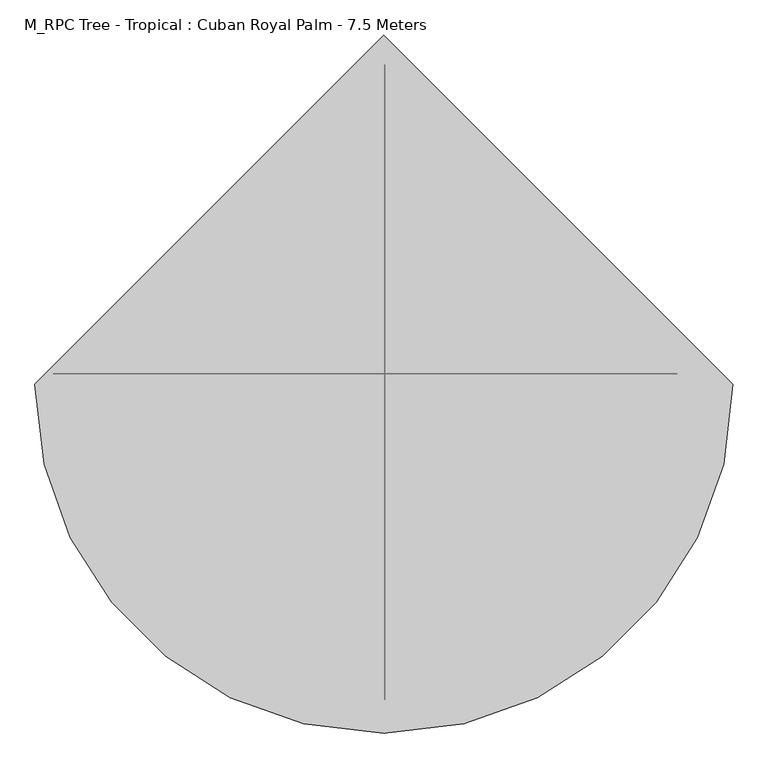
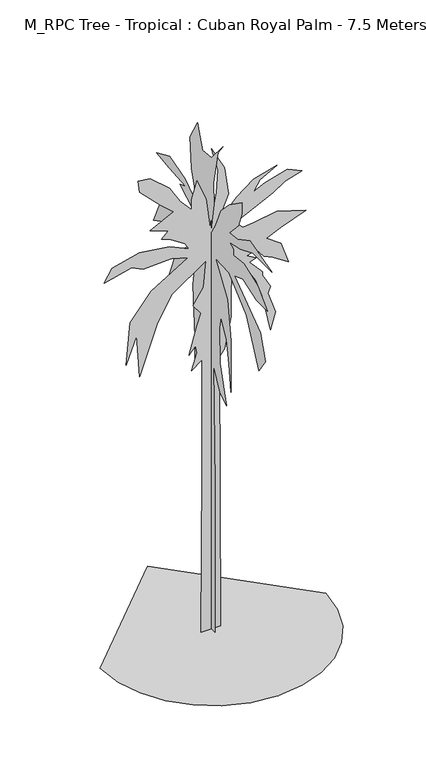
"""IFC4 building model written with IfcOpenShell, lengths in millimetres: geographic element geometry, M_RPC Tree - Tropical : Cuban Royal Palm - 7.5 Meters."""

from ifc_helpers import new_model, si_unit, origin, place, context, project, spatial, triangles, source, transform, mapped, element, save


def m_rpc_tree_tropical_cuban_royal_palm_7_5_meters_87faf919(model_context):
    return source(origin(), model_context, "Body", "Tessellation", [
        triangles([(-53.3295255, -0.0172155, 0.0009289), (-147.4824313, -0.0172239, 0.000933), (-128.6516948, -0.0176557, 2455.3626274), (-128.6514496, -0.0179554, 4131.270797), (-279.2955611, -0.0179286, 4018.2960068), (-203.9743774, -0.0179756, 4263.0955994), (-222.804369, -0.017995, 4376.0706802), (-316.9580152, -0.0179707, 4263.0955994), (-203.9741412, -0.0180497, 4677.3703125), (-147.482177, -0.0180825, 4846.8451424), (-260.4655695, -0.0181045, 4997.4949585), (-109.8212218, -0.0181515, 5223.4445389), (-72.1600077, -0.0182238, 5618.8942383), (-561.755246, -0.0181418, 5279.9445786), (-768.8900591, -0.0180688, 4922.1699051), (-1032.519825, -0.017926, 4187.7708366), (-1070.1798082, -0.0180388, 4828.0201286), (-1220.8246101, -0.0179615, 4432.5704292), (-1164.3346716, -0.0180751, 5053.9699997), (-863.0449951, -0.0181556, 5430.5946854), (-335.7879704, -0.0182359, 5750.7193314), (-580.5852376, -0.0182387, 5826.0443848), (-976.027343, -0.018218, 5807.1943726), (-1145.5022455, -0.0182241, 5882.5188446), (-1540.9443146, -0.0181899, 5788.3693588), (-1427.9619667, -0.0182286, 5976.6689117), (-1032.519825, -0.0182627, 6070.8439774), (-599.4152292, -0.0182715, 6014.3439377), (-316.9580152, -0.0182603, 5882.5188446), (-373.4504608, -0.0182746, 5976.6689117), (-599.4152292, -0.0182917, 6127.3190186), (-712.4001205, -0.0182935, 6164.9940445), (-618.247728, -0.0183145, 6259.1435303), (-881.8749504, -0.0183198, 6353.2935974), (-542.9252907, -0.0183649, 6522.768718), (-731.2301485, -0.018387, 6692.2432571), (-1032.519825, -0.0184277, 6993.5428894), (-1051.3497803, -0.0184571, 7163.0180099), (-881.8749504, -0.0184612, 7144.1679977), (-599.4152292, -0.0184298, 6899.3678238), (-448.7703547, -0.0183926, 6654.5682312), (-279.2955611, -0.0183663, 6466.2686783), (-279.2955611, -0.0183932, 6616.9182037), (-203.9741412, -0.0184437, 6880.5433914), (-72.1600077, -0.0183922, 6560.4181641), (-15.6683375, -0.0183139, 6108.4940048), (78.4845898, -0.0184055, 6598.09319), (97.3153263, -0.018467, 6937.0428497), (3.162393, -0.0185268, 7294.8175232), (191.4682185, -0.0184711, 6937.0428497), (247.9601737, -0.0183995, 6522.768718), (78.4845898, -0.018318, 6108.4940048), (360.9438114, -0.0183876, 6428.6186508), (605.7410786, -0.0184319, 6616.9182037), (944.6906656, -0.0184636, 6711.0682709), (699.8934711, -0.0184293, 6579.2681763), (605.7410786, -0.0183983, 6428.6186508), (775.2158358, -0.0184191, 6503.9437042), (1095.3355402, -0.01845, 6598.09319), (1302.4728241, -0.0184422, 6503.9437042), (1057.6755569, -0.018418, 6428.6186508), (888.2007271, -0.0183904, 6315.6185715), (342.1138561, -0.0183194, 6051.9939651), (455.0962403, -0.0183041, 5939.0188843), (605.7410786, -0.0183141, 5957.843898), (944.6906656, -0.018339, 6014.3439377), (1358.9653061, -0.0183335, 5882.5188446), (1001.1831476, -0.0182943, 5750.7193314), (794.0458637, -0.0182684, 5656.5692642), (1001.1831476, -0.0182506, 5505.9197388), (1114.1654955, -0.0181983, 5185.7950928), (888.2007271, -0.0182153, 5336.4446182), (756.3858805, -0.0182197, 5392.9196594), (605.7410786, -0.0182467, 5581.2442108), (605.7410786, -0.0182366, 5524.7447525), (511.588686, -0.0182258, 5487.094725), (643.4009892, -0.0182181, 5411.7696716), (549.2486329, -0.0182072, 5374.0946457), (737.5559252, -0.0181784, 5166.970079), (737.5559252, -0.0181683, 5110.4700394), (850.538273, -0.0181362, 4903.3448914), (812.8783625, -0.0181177, 4809.1951149), (925.8607103, -0.0180654, 4489.0704689), (850.538273, -0.0180184, 4244.2708763), (737.5559252, -0.0181111, 4790.3451027), (643.4009892, -0.0181575, 5072.8200119), (473.9261956, -0.0182006, 5355.269632), (304.4513658, -0.0182066, 5430.5946854), (285.6213741, -0.0181385, 5053.9699997), (285.6213741, -0.0180644, 4639.720285), (191.4682185, -0.0179795, 4187.7708366), (116.1458085, -0.0179593, 4093.6207695), (134.9762906, -0.0172295, 0.0009206), (0.1930215, 88.1876585, 0.0004872), (0.1930211, 161.0565937, 0.0005002), (0.1930215, 161.0565937, 1798.0107456), (0.1930235, 142.8396097, 4220.8958496), (0.1930219, 215.7080362, 4111.5958351), (0.1930238, 397.879602, 3729.0212219), (0.1930224, 397.879602, 4184.4707474), (0.1930226, 452.5320436, 4949.5949753), (0.1930212, 379.6621093, 5477.8947052), (0.1930204, 525.3994709, 5313.9198303), (0.1930227, 780.4417522, 4785.6201004), (0.1930231, 1071.9164028, 4421.295536), (0.193021, 1290.521228, 4075.1710236), (0.1930224, 1035.4814901, 4767.4203392), (0.193022, 871.5265995, 5168.1950043), (0.193022, 507.1819782, 5532.5442764), (0.1930205, 671.1367962, 5496.0947571), (0.1930222, 889.7440922, 5477.8947052), (0.1930219, 1090.1338955, 5514.3192261), (0.1930219, 1436.2610241, 5332.1448807), (0.1930208, 1254.0887135, 5732.9192551), (0.1930227, 1053.6989101, 5732.9192551), (0.1930224, 980.8290121, 6042.618956), (0.1930219, 634.7043543, 5969.7437531), (0.1930206, 416.0970946, 6079.0440582), (0.1930204, 780.4417522, 6279.443454), (0.1930236, 634.7043543, 6334.0936066), (0.1930213, 1035.4814901, 6370.5187088), (0.193023, 1363.3911987, 6406.9688095), (0.1930222, 1035.4814901, 6552.6936356), (0.193022, 652.921847, 6443.3933304), (0.1930203, 343.2271603, 6224.7938828), (0.1930224, 488.967029, 6698.4434601), (0.1930226, 525.3994709, 7153.8679871), (0.1930219, 343.2271603, 7481.7677399), (0.1930226, 306.794682, 7372.4674347), (0.1930225, 215.7080362, 7135.6429367), (0.1930209, -2.898197, 7153.8679871), (0.1930232, -294.3722026, 7499.9927902), (0.1930217, -166.8530786, 7336.0429138), (0.1930211, -57.549694, 6807.7431839), (0.193021, -75.7669232, 6498.043483), (0.1930205, 15.3189596, 5987.9688034), (0.1930237, -112.2016361, 6188.343782), (0.1930209, -239.7217594, 6498.043483), (0.1930209, -458.3270388, 6716.643512), (0.1930205, -768.0192547, 6935.2679581), (0.1930205, -768.0192547, 6771.2930832), (0.1930212, -676.9343348, 6534.4935837), (0.1930204, -458.3270388, 6297.6685043), (0.1930231, -658.7168421, 6315.8685562), (0.1930203, -968.409058, 6479.8184326), (0.193022, -1514.9259899, 6334.0936066), (0.1930214, -1041.278956, 6334.0936066), (0.1930223, -731.5867401, 6206.5688324), (0.1930212, -458.3270388, 6151.9186798), (0.1930219, -549.4144658, 6097.2691086), (0.1930215, -549.4144658, 6006.1938538), (0.1930218, -822.67166, 6042.618956), (0.1930224, -1168.7988613, 5915.0941818), (0.193023, -1405.6210339, 5678.2691025), (0.1930208, -1132.363876, 5678.2691025), (0.1930229, -786.2367474, 5787.5694077), (0.1930214, -585.8494148, 5714.7192032), (0.1930226, -1223.4513393, 5241.0696259), (0.1930224, -1350.971172, 4876.720063), (0.1930228, -1187.0162813, 4639.8952744), (0.1930223, -877.3241381, 5295.7197784), (0.1930226, -440.1120532, 5678.2691025), (0.1930235, -112.2016361, 5696.4941528), (0.1930228, -403.6771042, 5241.0696259), (0.1930226, -494.7619878, 4676.3203766), (0.1930204, -494.7619878, 3892.9960968), (0.1930225, -440.1120532, 4293.7707619), (0.1930215, -385.4596115, 4621.6705147), (0.1930212, -239.7217594, 4876.720063), (0.1930219, -203.2873009, 4694.5454269), (0.1930229, -221.504521, 4166.245697), (0.1930203, -385.4596115, 3619.7214981), (0.1930216, -221.504521, 3729.0212219), (0.1930209, -57.549694, 4038.7209229), (0.1930231, -93.9844068, 2253.4402142), (0.1930206, -93.9844068, 0.0004546), (-1626.8666862, -48.3554514, 0.0005339), (-1583.9693047, -420.1520797, 0.0004655), (-1461.7994362, -761.5892693, 0.0003991), (-1270.1396233, -1062.88396, 0.0003369), (-1018.7723356, -1314.2511749, 0.0002809), (-717.4776449, -1505.9109879, 0.0002335), (-376.0429261, -1628.0808563, 0.0001967), (-4.2444496, -1670.9783833, 0.0001728), (367.5538004, -1628.0808563, 0.0001642), (708.9884102, -1505.9109879, 0.0001711), (1010.2831009, -1314.2511749, 0.0001922), (1261.6503159, -1062.88396, 0.0002262), (1453.3101288, -761.5892693, 0.0002717), (1575.4799973, -420.1520797, 0.0003274), (1618.3775242, -48.3554514, 0.000392), (-4.2447494, 1574.2659725, 0.000298)], [[54, 55, 56], [48, 49, 50], [17, 18, 19], [15, 16, 17], [7, 8, 9], [83, 84, 85], [82, 83, 85], [4, 5, 6], [70, 71, 72], [66, 67, 68], [43, 44, 45], [59, 60, 61], [24, 25, 26], [24, 26, 27], [33, 34, 35], [76, 77, 78], [58, 59, 61], [58, 61, 62], [31, 32, 33], [42, 43, 45], [42, 45, 46], [37, 38, 39], [54, 56, 57], [53, 54, 57], [23, 24, 27], [23, 27, 28], [22, 23, 28], [22, 28, 29], [21, 22, 29], [58, 62, 63], [57, 58, 63], [53, 57, 63], [52, 53, 63], [36, 37, 39], [36, 39, 40], [36, 40, 41], [35, 36, 41], [35, 41, 42], [69, 70, 72], [69, 72, 73], [69, 73, 74], [65, 66, 68], [65, 68, 69], [65, 69, 74], [64, 65, 74], [47, 48, 50], [47, 50, 51], [46, 47, 51], [46, 51, 52], [33, 35, 42], [82, 85, 86], [81, 82, 86], [80, 81, 86], [33, 42, 46], [31, 33, 46], [30, 31, 46], [29, 30, 46], [15, 17, 19], [15, 19, 20], [14, 15, 20], [14, 20, 21], [13, 14, 21], [92, 93, 1], [92, 1, 2], [92, 2, 3], [92, 3, 4], [80, 86, 87], [79, 80, 87], [78, 79, 87], [76, 78, 87], [76, 87, 88], [13, 21, 29], [13, 29, 46], [13, 46, 52], [13, 52, 63], [13, 63, 64], [13, 64, 74], [13, 74, 75], [13, 75, 76], [13, 76, 88], [12, 13, 88], [12, 88, 89], [11, 12, 89], [10, 11, 89], [10, 89, 90], [9, 10, 90], [9, 90, 91], [7, 9, 91], [6, 7, 91], [4, 6, 91], [92, 4, 91], [131, 132, 133], [165, 166, 167], [105, 106, 107], [145, 146, 147], [165, 167, 168], [98, 99, 100], [131, 133, 134], [121, 122, 123], [104, 105, 107], [112, 113, 114], [171, 172, 173], [171, 173, 174], [153, 154, 155], [127, 128, 129], [118, 119, 120], [112, 114, 115], [139, 140, 141], [139, 141, 142], [159, 160, 161], [158, 159, 161], [157, 158, 161], [157, 161, 162], [104, 107, 108], [103, 104, 108], [103, 108, 109], [102, 103, 109], [127, 129, 130], [121, 123, 124], [120, 121, 124], [120, 124, 125], [118, 120, 125], [153, 155, 156], [152, 153, 156], [151, 152, 156], [151, 156, 157], [126, 127, 130], [145, 147, 148], [144, 145, 148], [144, 148, 149], [143, 144, 149], [139, 142, 143], [138, 139, 143], [137, 138, 143], [137, 143, 149], [175, 176, 94], [175, 94, 95], [175, 95, 96], [175, 96, 97], [174, 175, 97], [111, 112, 115], [115, 116, 117], [111, 115, 117], [110, 111, 117], [109, 110, 117], [165, 168, 169], [164, 165, 169], [130, 131, 134], [126, 130, 134], [126, 134, 135], [125, 126, 135], [125, 135, 136], [118, 125, 136], [151, 157, 162], [171, 174, 97], [170, 171, 97], [109, 117, 118], [109, 118, 136], [102, 109, 136], [97, 98, 100], [97, 100, 101], [170, 97, 101], [169, 170, 101], [169, 101, 102], [164, 169, 102], [163, 164, 102], [163, 102, 136], [151, 162, 163], [151, 163, 136], [151, 136, 137], [151, 137, 149], [151, 149, 150], [191, 192, 177], [190, 191, 177], [190, 177, 178], [189, 190, 178], [189, 178, 179], [189, 179, 180], [188, 189, 180], [187, 188, 180], [187, 180, 181], [187, 181, 182], [187, 182, 183], [187, 183, 184], [187, 184, 185], [187, 185, 186]], closed=False),
    ])


if __name__ == "__main__":
    model = new_model("IFC4")
    model_context = context("Model", 3, world=origin())
    ifc_project = project(units=[si_unit("LENGTHUNIT", "METRE", prefix="MILLI")], contexts=[model_context])
    site = spatial("IfcSite", under=ifc_project)
    building = spatial("IfcBuilding", under=site)
    placement = place(None, origin())
    m_rpc_tree_tropical_cuban_royal_palm_7_5_meters_shape = m_rpc_tree_tropical_cuban_royal_palm_7_5_meters_87faf919(model_context)
    element("IfcGeographicElement", 1, ObjectType="M_RPC Tree - Tropical : Cuban Royal Palm - 7.5 Meters", at=placement, inside=building, context=model_context, shape_type="MappedRepresentation", body=[
        mapped(m_rpc_tree_tropical_cuban_royal_palm_7_5_meters_shape, transform((0.0, 0.0, 0.0), x_axis=(1.0, 0.0, 0.0), y_axis=(0.0, 1.0, 0.0), z_axis=(0.0, 0.0, 1.0))),
    ])
    save(model, "model.ifc")

# Revit data of these elements
# Type "M_RPC Tree - Tropical : Cuban Royal Palm - 7.5 Meters"
#   built-in parameter 1005198 = "{2, 15},{39, RPC-16-FVGV-NKG0-7NHH-C000-ST1L-LVER-AU},{1, 0},{1, 0},{2, 35},{1, 8},{5, Color},{1, 0},{1, 0},{3, 0.8},{3, 0.8},{3, 0.8},{1, 8},{7, BBoxMin},{1, 0},{1, 0},{1, 0},{1, 0},{1, 0},{1, 8},{7, BBoxMax},{1, 0},{1, 0},{1, 0},{1, 0},{1, 0},{2, 11},{9, RPCTypeId},{1, 0},{1, 0},{39, RPC-16-FVGV-NKG0-7NHH-C000-ST1L-LVER-AU},{1, 6},{14, RPCPlantHeight},{1, 0},{1, 0},{7, 24.6063},{2, 11},{7, keyword},{1, 0},{1, 0},{72, :Geometry:RPC:Cuban Royal Palm:Roystonea regia (Oreodoxa):palm:tropical.},{2, 11},{8, category},{1, 0},{1, 0},{17, :Trees [Tropical]},{2, 11},{12, LocalizedUID},{1, 0},{1, 0},{16, Cuban Royal Palm},{2, 14},{6, Height},{1, 0},{1, 0},{7, 24.6063},{1, 2},{16, Cast Reflections},{1, 0},{1, 0},{1, 0},{1, 2},{12, Cast Shadows},{1, 0},{1, 0},{1, 1},{1, 2},{9, Lock View},{1, 0},{1, 0},{1, 0},{1, 4},{5, ViewC},{1, 0},{1, 0},{1, 0},{2, 11},{20, AdvancedUIDefinition},{1, 0},{1, 0},{0, },{2, 11},{10, AssetLibID},{1, 0},{1, 0},{36, 4D3F6E72-3F99-4203-98E9-AF80B3C7A7A4},{2, 11},{10, BaseSchema},{1, 0},{1, 0},{9, RPCSchema},{2, 11},{12, ExchangeGUID},{1, 0},{1, 0},{0, },{1, 2},{6, Hidden},{1, 0},{1, 0},{1, 0},{1, 4},{11, RPCCategory},{1, 0},{1, 0},{1, 0},{2, 11},{8, RPCImage},{1, 0},{1, 0},{0, },{1, 4},{13, SchemaVersion},{1, 0},{1, 0},{1, 4},{2, 11},{12, UIDefinition},{1, 0},{1, 0},{0, },{2, 11},{6, UIName},{1, 0},{1, 0},{39, RPC-16-FVGV-NKG0-7NHH-C000-ST1L-LVER-AU},{2, 11},{11, VersionGUID},{1, 0},{1, 0},{9, RPCSchema},{2, 11},{9, assettype},{1, 0},{1, 0},{11, RPCGeometry},{2, 11},{11, description},{1, 0},{1, 0},{0, },{2, 11},{9, localname},{1, 0},{1, 0},{3, RPC},{2, 11},{9, localtype},{1, 0},{1, 0},{3, RPC},{1, 4},{8, revision},{1, 0},{1, 0},{1, 1},{2, 11},{9, thumbnail},{1, 0},{1, 0},{0, },{1, 4},{7, version},{1, 0},{1, 0},{1, 1},{1, 2},{20, RPC_Cast Reflections},{1, 0},{1, 0},{1, 1},{1, 2},{16, RPC_Cast Shadows},{1, 0},{1, 0},{1, 1},{1, 2},{13, RPC_Lock View},{1, 0},{1, 0},{1, 0},{1, 4},{9, RPC_ViewC},{1, 0},{1, 0},{1, 0},{21, assetlibrary_base.fbx},{1, 5},"
#   built-in parameter 1005195 = "RPC-16-FVGV-NKG0-7NHH-C000-ST1L-LVER-AU"
#   Type Comments = "Cuban Royal Palm"
#   Height = 7500 mm
#   Plan Symbol = element 405753
#   Description = (empty or 0)
#   Default Elevation = 0
